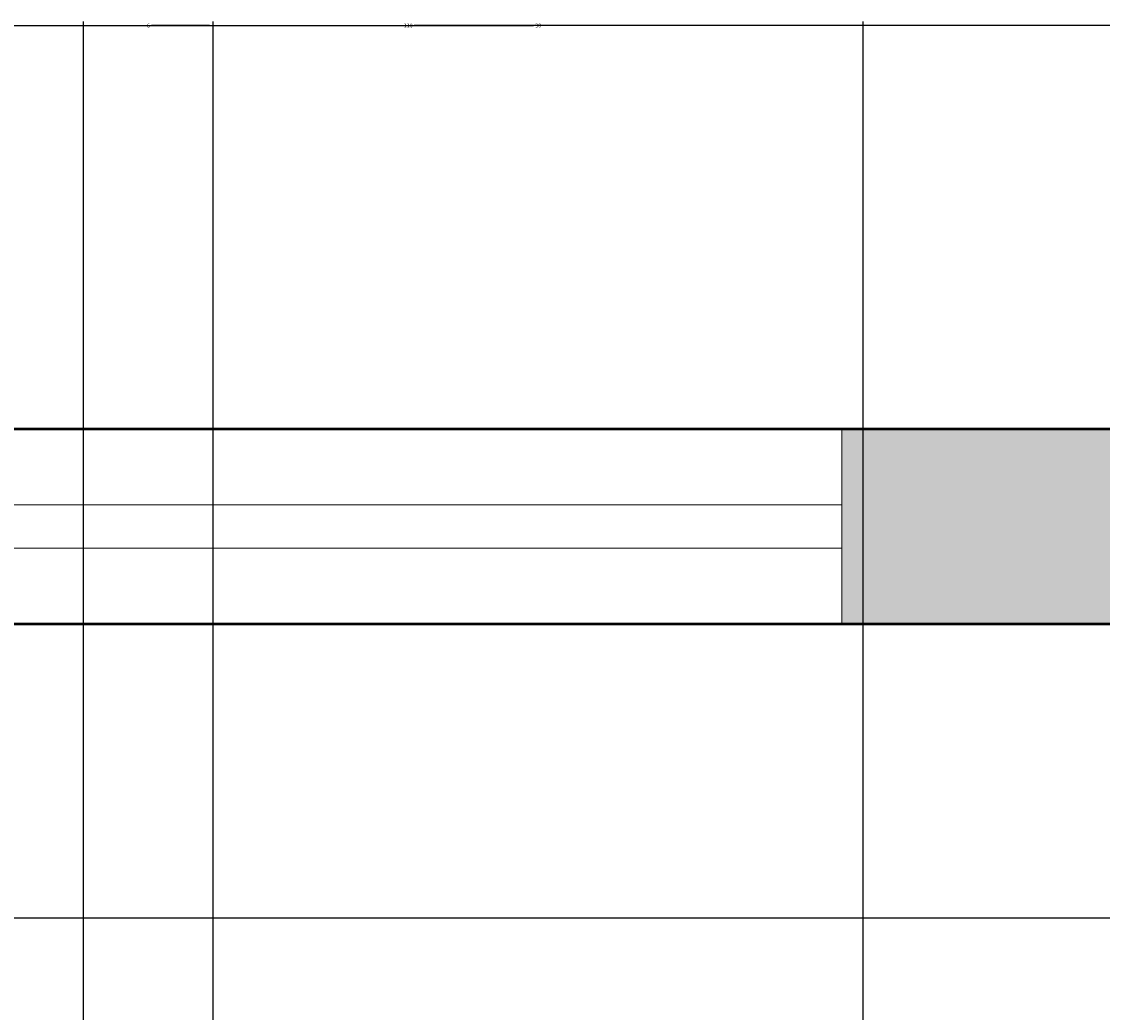
# Model space of a CAD drawing. Units: inches. Extents: x 2231 to 2461, y 2045 to 2455.
# Tile 78 of 95: x 2296 to 2346, y 2409 to 2455. Entities that reach past the tile are written whole.
import ezdxf

# ---------------------------------------------------------------- set-up
doc = ezdxf.new("R2010")
doc.units = ezdxf.units.IN
for name, color, linetype, lineweight in [('A-ANNO-DIMS', 2, 'Continuous', 18), ('A-GLAZ', 4, 'Continuous', 18), ('A-WALL', 7, 'Continuous', 50)]:
    doc.layers.add(name, color=color, linetype=linetype, lineweight=lineweight)
doc.layers.add('A-WALL-PATT', color=18, linetype='Continuous', lineweight=13, true_color=0x000000)
doc.styles.get("Standard").update_dxf_attribs({"font": 'arial.ttf'})
doc.dimstyles.get("Standard").update_dxf_attribs({"dimtxt": 0.18, "dimasz": 0.18, "dimexe": 0.18, "dimexo": 0.0625, "dimgap": 0.09, "dimtad": 0, "dimtih": 1, "dimtoh": 1, "dimdec": 4, "dimzin": 0, "dimdsep": 46, "dimtxsty": 'Standard', "dimcen": 0.09, "dimadec": 0, "dimazin": 0, "dimtfac": 1, "dimtdec": 4, "dimtofl": 0, "dimtmove": 0, "dimatfit": 3, "dimfxl": 1, "dimtolj": 1, "dimtzin": 0, "dimarcsym": 0})

# ---------------------------------------------------------------- blocks, each defined once
blk = doc.blocks.new('WIN-48IN')
for p, q in [((0, 0), (0, 9)), ((48, 9), (48, 0)), ((0, 5.5), (48, 5.5)), ((0, 3.5), (48, 3.5))]:
    blk.add_line(p, q)
blk = doc.blocks.new('*D35')
at = {"layer": 'A-ANNO-DIMS', "color": 0, "lineweight": -2, "transparency": 16777216}
for p, q in [((2258.794, 2426.895), (2258.794, 2454.645)), ((2258.974, 2454.465), (2313.513, 2454.465)), ((2368.614, 2454.465), (2314.074, 2454.465)), ((2368.794, 2426.895), (2368.794, 2454.645))]:
    blk.add_line(p, q, dxfattribs=at)
at = {"layer": 'A-ANNO-DIMS', "color": 0, "transparency": 16777216}
for points in [[(2258.974, 2454.495), (2258.974, 2454.435), (2258.794, 2454.465)], [(2368.614, 2454.495), (2368.614, 2454.435), (2368.794, 2454.465)]]:
    blk.add_solid(points, dxfattribs=at)
at = {"layer": 'Defpoints', "color": 0, "transparency": 16777216}
for p in [(2368.794, 2454.465), (2258.794, 2426.833), (2368.794, 2426.833)]:
    blk.add_point(p, dxfattribs=at)
at = {"layer": 'A-ANNO-DIMS', "color": 0, "transparency": 16777216, "insert": (2313.794, 2454.465), "char_height": 0.18, "attachment_point": 5}
blk.add_mtext('\\A1;110', dxfattribs=at)
blk = doc.blocks.new('*D49')
at = {"layer": 'A-ANNO-DIMS', "color": 0, "lineweight": -2, "transparency": 16777216}
for p, q in [((2298.794, 2182.895), (2298.794, 2454.645)), ((2298.974, 2454.465), (2301.644, 2454.465)), ((2304.614, 2454.465), (2301.943, 2454.465)), ((2304.794, 2182.895), (2304.794, 2454.645))]:
    blk.add_line(p, q, dxfattribs=at)
at = {"layer": 'A-ANNO-DIMS', "color": 0, "transparency": 16777216}
for points in [[(2298.974, 2454.495), (2298.974, 2454.435), (2298.794, 2454.465)], [(2304.614, 2454.495), (2304.614, 2454.435), (2304.794, 2454.465)]]:
    blk.add_solid(points, dxfattribs=at)
at = {"layer": 'Defpoints', "color": 0, "transparency": 16777216}
for p in [(2304.794, 2454.465), (2298.794, 2182.833), (2304.794, 2182.833)]:
    blk.add_point(p, dxfattribs=at)
at = {"layer": 'A-ANNO-DIMS', "color": 0, "transparency": 16777216, "insert": (2301.794, 2454.465), "char_height": 0.18, "attachment_point": 5}
blk.add_mtext('\\A1;6', dxfattribs=at)
blk = doc.blocks.new('*D50')
at = {"layer": 'A-ANNO-DIMS', "color": 0, "lineweight": -2, "transparency": 16777216}
for p, q in [((2304.794, 2182.895), (2304.794, 2454.645)), ((2304.974, 2454.465), (2319.575, 2454.465)), ((2334.614, 2454.465), (2320.012, 2454.465)), ((2334.794, 2182.895), (2334.794, 2454.645))]:
    blk.add_line(p, q, dxfattribs=at)
at = {"layer": 'A-ANNO-DIMS', "color": 0, "transparency": 16777216}
for points in [[(2304.974, 2454.495), (2304.974, 2454.435), (2304.794, 2454.465)], [(2334.614, 2454.495), (2334.614, 2454.435), (2334.794, 2454.465)]]:
    blk.add_solid(points, dxfattribs=at)
at = {"layer": 'Defpoints', "color": 0, "transparency": 16777216}
for p in [(2334.794, 2454.465), (2304.794, 2182.833), (2334.794, 2182.833)]:
    blk.add_point(p, dxfattribs=at)
at = {"layer": 'A-ANNO-DIMS', "color": 0, "transparency": 16777216, "insert": (2319.794, 2454.465), "char_height": 0.18, "attachment_point": 5}
blk.add_mtext('\\A1;30', dxfattribs=at)
blk = doc.blocks.new('*D68')
at = {"layer": 'A-ANNO-DIMS', "color": 0, "lineweight": -2, "transparency": 16777216}
for p, q in [((2285.882, 2426.833), (2460.606, 2426.833)), ((2460.426, 2426.653), (2460.426, 2420.225)), ((2460.426, 2413.433), (2460.426, 2419.861)), ((2278.251, 2413.253), (2460.606, 2413.253))]:
    blk.add_line(p, q, dxfattribs=at)
at = {"layer": 'A-ANNO-DIMS', "color": 0, "transparency": 16777216}
for points in [[(2460.396, 2426.653), (2460.456, 2426.653), (2460.426, 2426.833)], [(2460.396, 2413.433), (2460.456, 2413.433), (2460.426, 2413.253)]]:
    blk.add_solid(points, dxfattribs=at)
at = {"layer": 'Defpoints', "color": 0, "transparency": 16777216}
for p in [(2285.82, 2426.833), (2460.426, 2426.833), (2278.188, 2413.253)]:
    blk.add_point(p, dxfattribs=at)
at = {"layer": 'A-ANNO-DIMS', "color": 0, "transparency": 16777216, "insert": (2460.426, 2420.043), "char_height": 0.18, "attachment_point": 5}
blk.add_mtext('\\A1;13.58', dxfattribs=at)

msp = doc.modelspace()

# ---------------------------------------------------------------- hatches: boundary and pattern name
at = {"layer": 'A-WALL-PATT'}
h = msp.add_hatch(color=256, dxfattribs=at)
h.dxf.hatch_style = 1
h.paths.add_polyline_path([(2441.7935, 2269.1535), (2432.7935, 2269.1535), (2432.7935, 2186.8328), (2396.7935, 2186.8328), (2396.7935, 2286.8328), (2394.7935, 2286.8328), (2394.7935, 2186.8328), (2334.7935, 2186.8328), (2334.7935, 2182.8328), (2432.7935, 2182.8328), (2432.7935, 2072.8328), (2416.6639, 2072.8328), (2416.6639, 2063.8328), (2441.7935, 2063.8328)])
h.paths.add_polyline_path([(2368.6639, 2072.8328), (2367.04, 2072.8328), (2330.7942, 2072.8328), (2330.7397, 2063.8328), (2368.6639, 2063.8328)])
h.paths.add_polyline_path([(2300.7392, 2068.3328), (2300.7392, 2072.8328), (2298.7935, 2072.8328), (2294.7935, 2072.8328), (2258.7935, 2072.8328), (2258.7935, 2120.8328), (2294.7935, 2120.8328), (2298.7935, 2120.8328), (2298.7935, 2128.8328), (2294.7935, 2128.8328), (2294.7935, 2124.8328), (2258.7935, 2124.8328), (2258.7935, 2182.8328), (2294.7935, 2182.8328), (2294.7935, 2174.8328), (2298.7935, 2174.8328), (2298.7935, 2182.8328), (2304.7935, 2182.8328), (2304.7935, 2186.8328), (2258.7935, 2186.8328), (2258.7935, 2221.999), (2249.7935, 2221.999), (2249.7935, 2063.8328), (2300.7392, 2063.8328)])
h.paths.add_polyline_path([(2391.9338, 2435.8328), (2333.82, 2435.8328), (2333.82, 2426.8328), (2368.7935, 2426.8328), (2368.7935, 2374.9508), (2368.7935, 2370.8328), (2372.3935, 2370.8328), (2372.7935, 2370.8328), (2372.7935, 2426.8328), (2391.9338, 2426.8328)])
h.paths.add_polyline_path([(2441.7935, 2435.8328), (2415.9338, 2435.8328), (2415.9338, 2426.8328), (2432.7935, 2426.8328), (2432.7935, 2334.8328), (2372.7935, 2334.8328), (2372.7935, 2346.8328), (2368.7935, 2346.8328), (2368.7935, 2306.8328), (2360.7935, 2306.8328), (2360.7935, 2302.8328), (2368.7935, 2302.8328), (2372.7935, 2302.8328), (2372.7935, 2330.8328), (2432.7935, 2330.8328), (2432.7935, 2317.1535), (2441.7935, 2317.1535)])
h.paths.add_polyline_path([(2285.82, 2435.8328), (2249.7935, 2435.8328), (2249.7935, 2269.999), (2258.7935, 2269.999), (2258.7935, 2302.8328), (2318.8168, 2302.8328), (2330.7935, 2302.8328), (2330.7935, 2306.8328), (2258.7935, 2306.8328), (2258.7935, 2426.8328), (2285.82, 2426.8328)])

# ---------------------------------------------------------------- linework, layer by layer
at = {"layer": 'A-WALL'}
msp.add_line((2258.7935, 2426.8328), (2368.7935, 2426.8328), dxfattribs=at)
msp.add_lwpolyline([(2300.7392, 2063.8328), (2249.7935, 2063.8328), (2249.7935, 2435.8328), (2441.7935, 2435.8328), (2441.7935, 2063.8328), (2330.7397, 2063.8328)], dxfattribs=at)

# ---------------------------------------------------------------- block references
at = {"layer": 'A-GLAZ'}
msp.add_blockref('WIN-48IN', (2285.82, 2426.833), dxfattribs=at)

# ---------------------------------------------------------------- dimensions: what is measured, and where the dimension line sits
at = {"layer": 'A-ANNO-DIMS'}
for base, p1, p2, picture, middle in [((2368.7935, 2454.4653), (2258.7935, 2426.8328), (2368.7935, 2426.8328), '*D35', (2313.7935, 2454.4653)), ((2304.7935, 2454.4653), (2298.7935, 2182.8328), (2304.7935, 2182.8328), '*D49', (2301.7935, 2454.4653)), ((2334.7935, 2454.4653), (2304.7935, 2182.8328), (2334.7935, 2182.8328), '*D50', (2319.7935, 2454.4653))]:
    dim = msp.add_linear_dim(base=base, p1=p1, p2=p2, dimstyle='Standard', override={"dimdec": 0, "dimlfac": 1, "dimrnd": 0, "dimzin": 0, "dimdsep": 46, "dimlunit": 2}, dxfattribs=at)
    dim.commit()
    dim.dimension.update_dxf_attribs({"geometry": picture, "text_midpoint": middle})
dim = msp.add_linear_dim(base=(2460.426, 2426.8328), p1=(2278.1881, 2413.2534), p2=(2285.82, 2426.8328), angle=90, dimstyle='Standard', override={"dimdec": 2, "dimlfac": 1, "dimrnd": 0, "dimzin": 0, "dimdsep": 46, "dimlunit": 2}, dxfattribs=at)
dim.commit()
dim.dimension.update_dxf_attribs({"geometry": '*D68', "text_midpoint": (2460.426, 2420.0431)})

doc.saveas('drawing.dxf')
